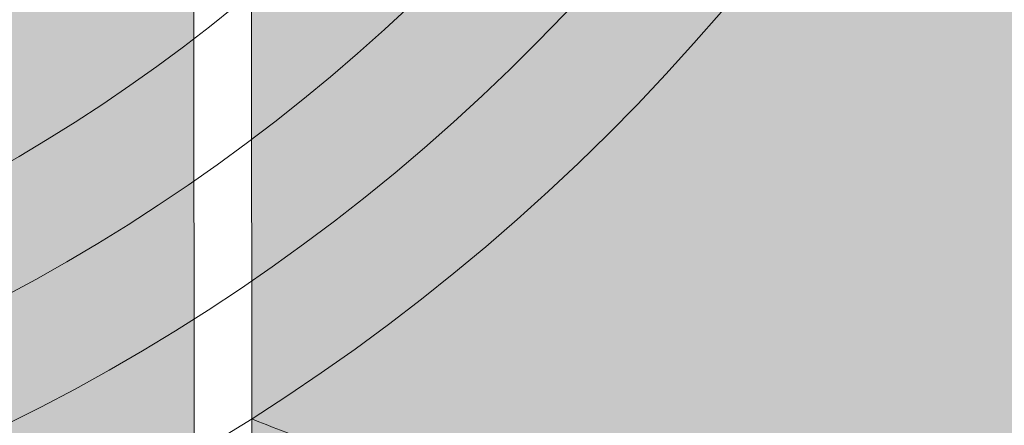
# Model space of a CAD drawing. Units: millimetres. Extents: x 11032 to 26788, y 3406 to 24505.
# Tile 23 of 78: x 18325 to 18753, y 10998 to 11174. Entities that reach past the tile are written whole.
import ezdxf

# ---------------------------------------------------------------- set-up
doc = ezdxf.new("R2010")
doc.units = ezdxf.units.MM
doc.header["$MEASUREMENT"] = 0
for name, color, linetype, lineweight in [('A-ANNO-DIMS', 2, 'Continuous', 18), ('A-ELEV-GUIT', 7, 'Continuous', 18), ('A-ELEV-GUIT-PATT', 7, 'Continuous', 13), ('A-ELEV-INLY', 8, 'Continuous', 13), ('A-ELEV-INLY-PATT', 250, 'Continuous', 13), ('A-ELEV-STRG', 7, 'Continuous', 13)]:
    doc.layers.add(name, color=color, linetype=linetype, lineweight=lineweight)
doc.styles.get("Standard").update_dxf_attribs({"font": 'arial.ttf'})
doc.dimstyles.get("Standard").update_dxf_attribs({"dimtxt": 150, "dimasz": 100, "dimexe": 10, "dimexo": 5, "dimgap": 5, "dimtad": 0, "dimtih": 1, "dimtoh": 1, "dimdec": 0, "dimzin": 0, "dimdsep": 46, "dimtxsty": 'Standard', "dimcen": 0.09, "dimadec": 0, "dimazin": 0, "dimtfac": 1, "dimtdec": 0, "dimtofl": 0, "dimtmove": 0, "dimatfit": 3, "dimfxl": 1, "dimtolj": 1, "dimtzin": 0, "dimarcsym": 0})

# ---------------------------------------------------------------- blocks, each defined once
blk = doc.blocks.new('*D36')
at = {"layer": 'A-ANNO-DIMS', "color": 0, "lineweight": -2, "transparency": 16777216}
for p, q in [((12301.26, 17115.89), (12301.26, 24416.86)), ((25397.4, 4466.4), (25397.4, 24416.86)), ((12401.26, 24406.86), (18569.2, 24406.86)), ((25297.4, 24406.86), (19129.47, 24406.86))]:
    blk.add_line(p, q, dxfattribs=at)
at = {"layer": 'A-ANNO-DIMS', "color": 0, "transparency": 16777216}
for points in [[(12401.26, 24423.52), (12401.26, 24390.19), (12301.26, 24406.86)], [(25297.4, 24423.52), (25297.4, 24390.19), (25397.4, 24406.86)]]:
    blk.add_solid(points, dxfattribs=at)
at = {"layer": 'Defpoints', "color": 0, "transparency": 16777216}
for p in [(25397.4, 24406.86), (12301.26, 17110.89), (25397.4, 4461.4)]:
    blk.add_point(p, dxfattribs=at)
at = {"layer": 'A-ANNO-DIMS', "color": 0, "transparency": 16777216, "insert": (18849.33, 24406.86), "char_height": 150, "attachment_point": 5}
blk.add_mtext('\\A1;13096', dxfattribs=at)
blk = doc.blocks.new('*D50')
at = {"layer": 'A-ANNO-DIMS', "color": 0, "lineweight": -2, "transparency": 16777216}
for p, q in [((19697.4, 16000.71), (19697.4, 3494.9)), ((17953.45, 10206.41), (17953.45, 3494.9)), ((18053.45, 3504.9), (18603.82, 3504.9)), ((19597.4, 3504.9), (19047.04, 3504.9))]:
    blk.add_line(p, q, dxfattribs=at)
at = {"layer": 'A-ANNO-DIMS', "color": 0, "transparency": 16777216}
for points in [[(18053.45, 3521.57), (18053.45, 3488.23), (17953.45, 3504.9)], [(19597.4, 3521.57), (19597.4, 3488.23), (19697.4, 3504.9)]]:
    blk.add_solid(points, dxfattribs=at)
at = {"layer": 'Defpoints', "color": 0, "transparency": 16777216}
for p in [(19697.4, 16005.71), (17953.45, 10211.41), (19697.4, 3504.9)]:
    blk.add_point(p, dxfattribs=at)
at = {"layer": 'A-ANNO-DIMS', "color": 0, "transparency": 16777216, "insert": (18825.43, 3504.9), "char_height": 150, "attachment_point": 5}
blk.add_mtext('\\A1;1744', dxfattribs=at)
blk = doc.blocks.new('*D57')
at = {"layer": 'A-ANNO-DIMS', "color": 0, "lineweight": -2, "transparency": 16777216}
for p, q in [((14994.7, 7266.4), (14994.7, 24416.86)), ((20894.7, 7266.4), (20894.7, 24416.86)), ((15094.7, 24406.86), (17715.98, 24406.86)), ((20794.7, 24406.86), (18173.42, 24406.86))]:
    blk.add_line(p, q, dxfattribs=at)
at = {"layer": 'A-ANNO-DIMS', "color": 0, "transparency": 16777216}
for points in [[(15094.7, 24423.52), (15094.7, 24390.19), (14994.7, 24406.86)], [(20794.7, 24423.52), (20794.7, 24390.19), (20894.7, 24406.86)]]:
    blk.add_solid(points, dxfattribs=at)
at = {"layer": 'Defpoints', "color": 0, "transparency": 16777216}
for p in [(20894.7, 24406.86), (14994.7, 7261.4), (20894.7, 7261.4)]:
    blk.add_point(p, dxfattribs=at)
at = {"layer": 'A-ANNO-DIMS', "color": 0, "transparency": 16777216, "insert": (17944.7, 24406.86), "char_height": 150, "attachment_point": 5}
blk.add_mtext('\\A1;5900', dxfattribs=at)
blk = doc.blocks.new('*D70')
at = {"layer": 'A-ANNO-DIMS', "color": 0, "lineweight": -2, "transparency": 16777216}
for p, q in [((18044.7, 11901.4), (17944.7, 11901.4)), ((17944.7, 11901.4), (17944.7, 10261.4)), ((17944.61, 7261.4), (17944.79, 7261.4)), ((17944.7, 7261.31), (17944.7, 7261.49))]:
    blk.add_line(p, q, dxfattribs=at)
at = {"layer": 'A-ANNO-DIMS', "color": 0, "transparency": 16777216}
blk.add_solid([(17928.04, 10261.4), (17961.37, 10261.4), (17944.7, 10161.4)], dxfattribs=at)
at = {"layer": 'Defpoints', "color": 0, "transparency": 16777216}
for p in [(17944.7, 10161.4), (17944.7, 7261.4)]:
    blk.add_point(p, dxfattribs=at)
at = {"layer": 'A-ANNO-DIMS', "color": 0, "transparency": 16777216, "insert": (18345.2, 11901.4), "char_height": 150, "attachment_point": 5}
blk.add_mtext('\\A1;R2900', dxfattribs=at)
blk = doc.blocks.new('*D78')
at = {"layer": 'A-ANNO-DIMS', "color": 0, "lineweight": -2, "transparency": 16777216}
for p, q in [((19278.06, 11833.8), (19378.06, 11833.8)), ((19378.06, 11833.8), (19386.9, 11238.32)), ((19405.52, 9979.24), (19405.7, 9979.24)), ((19405.61, 9979.15), (19405.61, 9979.33))]:
    blk.add_line(p, q, dxfattribs=at)
at = {"layer": 'A-ANNO-DIMS', "color": 0, "transparency": 16777216}
blk.add_solid([(19403.57, 11238.57), (19370.24, 11238.08), (19388.39, 11138.34)], dxfattribs=at)
at = {"layer": 'Defpoints', "color": 0, "transparency": 16777216}
for p in [(19388.39, 11138.34), (19405.61, 9979.24)]:
    blk.add_point(p, dxfattribs=at)
at = {"layer": 'A-ANNO-DIMS', "color": 0, "transparency": 16777216, "insert": (18728.26, 11833.8), "char_height": 150, "attachment_point": 5}
blk.add_mtext('\\A1;2X R1159.2', dxfattribs=at)
blk = doc.blocks.new('*D79')
at = {"layer": 'A-ANNO-DIMS', "color": 0, "lineweight": -2, "transparency": 16777216}
for p, q in [((19621.6, 11163.41), (19157.07, 10798.82)), ((19721.6, 11163.41), (19621.6, 11163.41)), ((18173, 10026.54), (18173.18, 10026.54)), ((18173.09, 10026.45), (18173.09, 10026.63))]:
    blk.add_line(p, q, dxfattribs=at)
at = {"layer": 'A-ANNO-DIMS', "color": 0, "transparency": 16777216}
blk.add_solid([(19146.78, 10811.93), (19167.36, 10785.71), (19078.4, 10737.08)], dxfattribs=at)
at = {"layer": 'Defpoints', "color": 0, "transparency": 16777216}
for p in [(19078.4, 10737.08), (18173.09, 10026.54)]:
    blk.add_point(p, dxfattribs=at)
at = {"layer": 'A-ANNO-DIMS', "color": 0, "transparency": 16777216, "insert": (20272.31, 11163.41), "char_height": 150, "attachment_point": 5}
blk.add_mtext('\\A1;2X R1150.9', dxfattribs=at)
blk = doc.blocks.new('*D80')
at = {"layer": 'A-ANNO-DIMS', "color": 0, "lineweight": -2, "transparency": 16777216}
for p, q in [((18808.09, 11500), (18908.09, 11500)), ((18908.09, 11500), (19122.53, 11163.36)), ((19623.1, 10377.38), (19623.28, 10377.38)), ((19623.19, 10377.29), (19623.19, 10377.47))]:
    blk.add_line(p, q, dxfattribs=at)
at = {"layer": 'A-ANNO-DIMS', "color": 0, "transparency": 16777216}
blk.add_solid([(19136.58, 11172.31), (19108.47, 11154.4), (19176.25, 11079.02)], dxfattribs=at)
at = {"layer": 'Defpoints', "color": 0, "transparency": 16777216}
for p in [(19176.25, 11079.02), (19623.19, 10377.38)]:
    blk.add_point(p, dxfattribs=at)
at = {"layer": 'A-ANNO-DIMS', "color": 0, "transparency": 16777216, "insert": (18315.64, 11500), "char_height": 150, "attachment_point": 5}
blk.add_mtext('\\A1;2X R831.9', dxfattribs=at)
blk = doc.blocks.new('*D81')
at = {"layer": 'A-ANNO-DIMS', "color": 0, "lineweight": -2, "transparency": 16777216}
for p, q in [((18746.01, 11278.33), (18846.01, 11278.33)), ((18846.01, 11278.33), (19073.46, 10960.86)), ((19607.77, 10214.96), (19607.95, 10214.96)), ((19607.86, 10214.87), (19607.86, 10215.05))]:
    blk.add_line(p, q, dxfattribs=at)
at = {"layer": 'A-ANNO-DIMS', "color": 0, "transparency": 16777216}
blk.add_solid([(19087.01, 10970.56), (19059.91, 10951.15), (19131.7, 10879.56)], dxfattribs=at)
at = {"layer": 'Defpoints', "color": 0, "transparency": 16777216}
for p in [(19131.7, 10879.56), (19607.86, 10214.96)]:
    blk.add_point(p, dxfattribs=at)
at = {"layer": 'A-ANNO-DIMS', "color": 0, "transparency": 16777216, "insert": (18253.76, 11278.33), "char_height": 150, "attachment_point": 5}
blk.add_mtext('\\A1;2X R817.6', dxfattribs=at)
blk = doc.blocks.new('*D83')
at = {"layer": 'A-ANNO-DIMS', "color": 0, "lineweight": -2, "transparency": 16777216}
for p, q in [((19272.33, 11150.07), (19043.23, 10964.72)), ((19372.33, 11150.07), (19272.33, 11150.07)), ((18454.06, 10487.99), (18454.06, 10488.17)), ((18453.97, 10488.08), (18454.15, 10488.08))]:
    blk.add_line(p, q, dxfattribs=at)
at = {"layer": 'A-ANNO-DIMS', "color": 0, "transparency": 16777216}
blk.add_solid([(19032.74, 10977.67), (19053.71, 10951.76), (18965.48, 10901.82)], dxfattribs=at)
at = {"layer": 'Defpoints', "color": 0, "transparency": 16777216}
for p in [(18965.48, 10901.82), (18454.06, 10488.08)]:
    blk.add_point(p, dxfattribs=at)
at = {"layer": 'A-ANNO-DIMS', "color": 0, "transparency": 16777216, "insert": (19864.78, 11150.07), "char_height": 150, "attachment_point": 5}
blk.add_mtext('\\A1;2X R657.8', dxfattribs=at)
blk = doc.blocks.new('*D84')
at = {"layer": 'A-ANNO-DIMS', "color": 0, "lineweight": -2, "transparency": 16777216}
for p, q in [((18888.04, 11434.41), (18988.04, 11434.41)), ((18988.04, 11434.41), (19243.8, 11304.14)), ((19907.6, 10966), (19907.78, 10966)), ((19907.69, 10965.91), (19907.69, 10966.09))]:
    blk.add_line(p, q, dxfattribs=at)
at = {"layer": 'A-ANNO-DIMS', "color": 0, "transparency": 16777216}
blk.add_solid([(19251.37, 11319), (19236.24, 11289.29), (19332.91, 11258.76)], dxfattribs=at)
at = {"layer": 'Defpoints', "color": 0, "transparency": 16777216}
for p in [(19332.91, 11258.76), (19907.69, 10966)]:
    blk.add_point(p, dxfattribs=at)
at = {"layer": 'A-ANNO-DIMS', "color": 0, "transparency": 16777216, "insert": (18482.56, 11434.41), "char_height": 150, "attachment_point": 5}
blk.add_mtext('\\A1;2X R645', dxfattribs=at)
blk = doc.blocks.new('*D85')
at = {"layer": 'A-ANNO-DIMS', "color": 0, "lineweight": -2, "transparency": 16777216}
for p, q in [((19336.15, 10949.98), (19136.5, 10931.99)), ((18538.07, 10878.07), (18538.25, 10878.07)), ((18538.16, 10877.98), (18538.16, 10878.16))]:
    blk.add_line(p, q, dxfattribs=at)
at = {"layer": 'A-ANNO-DIMS', "color": 0, "transparency": 16777216}
blk.add_solid([(19135, 10948.59), (19138, 10915.39), (19036.9, 10923.01)], dxfattribs=at)
at = {"layer": 'Defpoints', "color": 0, "transparency": 16777216}
for p in [(19036.9, 10923.01), (18538.16, 10878.07)]:
    blk.add_point(p, dxfattribs=at)
at = {"layer": 'A-ANNO-DIMS', "color": 0, "transparency": 16777216, "insert": (19828.6, 10949.98), "char_height": 150, "attachment_point": 5}
blk.add_mtext('\\A1;2X R500.8', dxfattribs=at)

msp = doc.modelspace()

# ---------------------------------------------------------------- hatches: boundary and pattern name
at = {"layer": 'A-ELEV-GUIT-PATT'}
h = msp.add_hatch(color=256, dxfattribs=at)
h.paths.add_polyline_path([(18424.39, 12337.941), (18425.299, 11185.614, 0.4683722)])
h.paths.add_polyline_path([(17502.928, 12367.48, 0.4909953), (17469.585, 11181.087)])
h.paths.add_polyline_path([(17654.236, 12452.868, 0.0477145), (17528.428, 12385.27), (17494.045, 11161.894, 0.0503453), (17622.952, 11083.922)])
h.paths.add_polyline_path([(17803.94, 12498.071, 0.0431928), (17679.468, 12462.933), (17647.696, 11072.715, 0.0458241), (17778.106, 11030.137)])
h.paths.add_polyline_path([(17950.249, 12511.239), (17829.354, 12521.528), (17803.014, 11024.905, 0.0436508), (17933.027, 11011.49)])
h.paths.add_polyline_path([(18101.906, 12494.739, 0.0426353), (17975.244, 12510.777), (17958.028, 11011.518, 0.0435176), (18087.619, 11025.142)])
h.paths.add_polyline_path([(18250.372, 12446.284, 0.0436439), (18126.849, 12488.945), (18112.671, 11030.45, 0.0462768), (18244.243, 11073.812)])
h.paths.add_polyline_path([(18399.373, 12357.869, 0.0487365), (18275.32, 12434.595), (18269.295, 11085.277, 0.0513698), (18400.312, 11165.647)])
h = msp.add_hatch(color=256, dxfattribs=at)
h.paths.add_polyline_path([(18424.244, 12523.003), (18424.291, 12463.18, -0.5273141), (18425.397, 11060.376), (18425.445, 11000.552, 0.5515566)])
h.paths.add_polyline_path([(18424.291, 12463.18), (18424.34, 12401.672, -0.4998624), (18425.349, 11121.884), (18425.397, 11060.376, 0.5273141)], flags=17)
h.paths.add_polyline_path([(18424.34, 12401.672), (18424.39, 12337.941, -0.4683722), (18425.299, 11185.614), (18425.349, 11121.884, 0.4998624)], flags=16)
h = msp.add_hatch(color=256, dxfattribs=at)
h.paths.add_polyline_path([(18400.408, 11043.88, -0.0436878), (18268.805, 10975.614), (18268.564, 10921.688, 0.0407453), (18400.454, 10985.325)])
h.paths.add_polyline_path([(18243.761, 10965.745, -0.0404734), (18111.675, 10927.96), (18111.179, 10876.93, 0.038119), (18243.523, 10912.454)])
h.paths.add_polyline_path([(18086.629, 10923.332, -0.0383771), (17956.879, 10911.486), (17956.305, 10861.474, 0.0362436), (18086.136, 10872.581)])
h.paths.add_polyline_path([(17931.879, 10911.496, -0.0386479), (17801.231, 10923.595), (17800.341, 10873.053, 0.0365688), (17931.305, 10861.499)])
h.paths.add_polyline_path([(17776.312, 10928.246, -0.0401698), (17645.255, 10965.893), (17644.048, 10913.103, 0.037865), (17775.419, 10877.463)])
h.paths.add_polyline_path([(17490.698, 11042.804), (17489.08, 10985.25, 0.0402314), (17619.258, 10922.301), (17620.478, 10975.665, -0.0430555)])
h.paths.add_polyline_path([(17492.349, 11101.569), (17490.698, 11042.804, 0.0430555), (17620.478, 10975.665), (17621.708, 11029.502, -0.0463742)])
h.paths.add_polyline_path([(17622.952, 11083.922, -0.0503453), (17494.045, 11161.894), (17492.349, 11101.569, 0.0463742), (17621.708, 11029.502)])
h.paths.add_polyline_path([(17647.696, 11072.715), (17646.47, 11019.067, 0.0427975), (17777.208, 10979.13), (17778.106, 11030.137, -0.0458241)])
h.paths.add_polyline_path([(17777.208, 10979.13, -0.0427975), (17646.47, 11019.067), (17645.255, 10965.893, 0.0401698), (17776.312, 10928.246)])
h.paths.add_polyline_path([(17932.453, 10961.493, -0.0409906), (17802.122, 10974.208), (17801.231, 10923.595, 0.0386479), (17931.879, 10911.496)])
h.paths.add_polyline_path([(17933.027, 11011.49, -0.0436508), (17803.014, 11024.905), (17802.122, 10974.208, 0.0409906), (17932.453, 10961.493)])
h.paths.add_polyline_path([(18087.619, 11025.142, -0.0435176), (17958.028, 11011.518), (17957.453, 10961.501, 0.040783), (18087.124, 10974.178)])
h.paths.add_polyline_path([(18087.124, 10974.178, -0.040783), (17957.453, 10961.501), (17956.879, 10911.486, 0.0383771), (18086.629, 10923.332)])
h.paths.add_polyline_path([(18243.761, 10965.745), (18244.001, 11019.495, -0.0431653), (18112.172, 10979.124), (18111.675, 10927.96, 0.0404734)])
h.paths.add_polyline_path([(18244.243, 11073.812, -0.0462768), (18112.671, 11030.45), (18112.172, 10979.124, 0.0431653), (18244.001, 11019.495)])
h.paths.add_polyline_path([(18400.361, 11103.846), (18400.312, 11165.647, -0.0513698), (18269.295, 11085.277), (18269.048, 11030.099, 0.0471686)])
h.paths.add_polyline_path([(18400.361, 11103.846, -0.0471686), (18269.048, 11030.099), (18268.805, 10975.614, 0.0436878), (18400.408, 11043.88)])
at = {"layer": 'A-ELEV-INLY-PATT'}
h = msp.add_hatch(color=256, dxfattribs=at)
h.set_gradient(color2=(38, 38, 39), name='HEMISPHERICAL')
edge = h.paths.add_edge_path()
edge.add_spline(control_points=[(18425.445, 11000.552), (18458.708, 10987.38), (18550.3, 10951.111), (18655.663, 10967.984), (18775.66, 10985.753), (18767.173, 11045.69), (18820.435, 11029.121), (18856.601, 11081.429), (18910.606, 10999.748), (18944.51, 11067.805), (18993.671, 11025.073), (19010.479, 11088.113), (19112.886, 11074.83), (18997.512, 11168.165), (19020.085, 11271.149), (19186.417, 11251.458), (19043.711, 11367.761), (19195.966, 11319.856), (19164.81, 11418.359), (19240.548, 11369.352), (19291.772, 11465.595), (19340.205, 11366.103), (19400.937, 11422.431), (19448.16, 11354.501), (19470.028, 11298.294), (19504.824, 11295.807)], knot_values=[0, 0, 0, 0, 104.1926844, 286.8965309, 358.0276019, 380.9077181, 428.8178922, 462.9108054, 536.6618053, 575.7062143, 616.0072998, 661.1892288, 710.1041052, 826.2545772, 880.3446099, 992.4558514, 1059.8900815, 1142.5885686, 1188.5458396, 1228.1561193, 1314.4611862, 1376.292047, 1433.035567, 1479.0146796, 1584.2445291, 1584.2445291, 1584.2445291, 1584.2445291], degree=3, periodic=0)
edge.add_spline(control_points=[(19504.824, 11295.807), (19505.924, 11314.349), (19506.623, 11332.908), (19508.291, 11422.259), (19504.403, 11492.427), (19485.077, 11629.54), (19469.639, 11696.485), (19436.971, 11793.081), (19424.498, 11824.643), (19403.303, 11870.856), (19395.824, 11886.073), (19380.021, 11916.101), (19371.692, 11930.911), (19325.511, 12008.031), (19280.532, 12066.689), (19204.455, 12147.807), (19177.661, 12173.701), (19101.242, 12241.001), (19049.213, 12279.949), (18967.517, 12332.138), (18939.676, 12348.496), (18883.071, 12379.019), (18854.309, 12393.182), (18810.69, 12412.702), (18796.068, 12418.926), (18764.062, 12431.927), (18746.648, 12438.606), (18662.541, 12469.232), (18594.628, 12489.063), (18492.28, 12515.967), (18458.285, 12524.419), (18424.236, 12532.741)], knot_values=[45.1275191, 45.1275191, 45.1275191, 45.1275191, 98.76835, 98.76835, 303.9642424, 303.9642424, 509.1601349, 509.1601349, 611.7580811, 611.7580811, 663.0570542, 663.0570542, 714.3560273, 714.3560273, 934.0138233, 934.0138233, 1043.8427213, 1043.8427213, 1233.750961, 1233.750961, 1328.7050808, 1328.7050808, 1423.6592007, 1423.6592007, 1471.1362606, 1471.1362606, 1527.0566313, 1527.0566313, 1739.8301307, 1739.8301307, 1844.9911016, 1844.9911016, 1844.9911016, 1844.9911016], degree=3, periodic=0)
edge.add_line((18424.236, 12532.741), (18424.244, 12523.003))
edge.add_arc((17944.704, 11761.399), 900, -57.713267, 57.803626, ccw=False)
h = msp.add_hatch(color=256, dxfattribs=at)
edge = h.paths.add_edge_path()
edge.add_line((18641.912, 10936.669), (18683.084, 10885.205))
edge.add_line((18683.084, 10885.205), (18707.528, 10942.241))
edge.add_line((18707.528, 10942.241), (18707.585, 10942.062))
edge.add_line((18707.585, 10942.062), (18728.977, 10934.931))
edge.add_line((18728.977, 10934.931), (18746.506, 10952.29))
edge.add_line((18746.506, 10952.29), (18731.852, 10933.973))
edge.add_line((18731.852, 10933.973), (18772.392, 10896.329))
edge.add_line((18772.392, 10896.329), (18806.063, 10924.18))
edge.add_line((18806.063, 10924.18), (18807.011, 10949.111))
edge.add_line((18807.011, 10949.111), (18828.079, 10974.85))
edge.add_line((18828.079, 10974.85), (18819.406, 10935.218))
edge.add_line((18819.406, 10935.218), (18806.063, 10924.18))
edge.add_line((18806.063, 10924.18), (18804.745, 10889.526))
edge.add_line((18804.745, 10889.526), (18898.625, 10928.045))
edge.add_line((18898.625, 10928.045), (18869.346, 10974.891))
edge.add_line((18869.346, 10974.891), (18881.224, 11043.454))
edge.add_spline(control_points=[(18881.224, 11043.454), (18869.883, 11051.959), (18847.69, 11068.541), (18820.435, 11029.121), (18767.173, 11045.69), (18775.66, 10985.753), (18655.663, 10967.984), (18550.3, 10951.111), (18458.708, 10987.38), (18425.445, 11000.552)], knot_values=[0, 0, 0, 0, 35.3761266, 69.4690398, 117.3792138, 140.25933, 211.3904011, 394.0942475, 498.2869319, 498.2869319, 498.2869319, 498.2869319], degree=3, periodic=0)
edge.add_line((18425.445, 11000.552), (18425.52, 10905.025))
edge.add_line((18425.52, 10905.025), (18430.245, 10896.05))
edge.add_line((18430.245, 10896.05), (18435.033, 10901.9))
edge.add_line((18435.033, 10901.9), (18426.36, 10862.267))
edge.add_line((18426.36, 10862.267), (18425.554, 10861.6))
edge.add_line((18425.554, 10861.6), (18425.592, 10814.001))
edge.add_spline(control_points=[(18425.592, 10814.001), (18433.789, 10803.871), (18442.268, 10794.033), (18451.048, 10784.539)], knot_values=[3268.8603349, 3268.8603349, 3268.8603349, 3268.8603349, 3307.7959894, 3307.7959894, 3307.7959894, 3307.7959894], degree=3, periodic=0)
edge.add_line((18451.048, 10784.539), (18509.494, 10848.83))
edge.add_line((18509.494, 10848.83), (18582.646, 10885.406))
edge.add_line((18582.646, 10885.406), (18583.089, 10886.145))
edge.add_line((18583.089, 10886.145), (18587.289, 10850.746))
edge.add_line((18587.289, 10850.746), (18609.162, 10818.698))
edge.add_line((18609.162, 10818.698), (18619.222, 10824.446))
edge.add_line((18619.222, 10824.446), (18621.931, 10828.059))
edge.add_line((18621.931, 10828.059), (18609.651, 10885.365))
edge.add_line((18609.651, 10885.365), (18631.427, 10872.922))
edge.add_line((18631.427, 10872.922), (18641.912, 10936.669))
edge = h.paths.add_edge_path()
edge.add_spline(control_points=[(18521.786, 10715.217), (18494.865, 10734.264), (18470.266, 10756.433), (18447.672, 10780.825)], knot_values=[3169.2083247, 3169.2083247, 3169.2083247, 3169.2083247, 3268.4288812, 3268.4288812, 3268.4288812, 3268.4288812], degree=3, periodic=0)
edge.add_line((18447.672, 10780.825), (18509.494, 10848.83))
edge.add_line((18509.494, 10848.83), (18553.129, 10870.647))
edge.add_line((18553.129, 10870.647), (18595.722, 10811.017))
edge.add_line((18595.722, 10811.017), (18533.878, 10775.678))
edge.add_line((18533.878, 10775.678), (18521.786, 10715.217))
h.paths.add_polyline_path([(18605.498, 10816.604), (18533.878, 10775.678), (18531.124, 10761.907), (18641.898, 10699.586), (18643.606, 10726.91), (18634.217, 10770.728)])
edge = h.paths.add_edge_path()
edge.add_line((18785.911, 10769.68), (18741.142, 10702.526))
edge.add_line((18741.142, 10702.526), (18708.511, 10675.334))
edge.add_line((18708.511, 10675.334), (18722.102, 10641.355))
edge.add_spline(control_points=[(18722.102, 10641.355), (18731.823, 10639.718), (18741.633, 10638.316), (18776.029, 10634.243), (18801.002, 10632.764), (18826.213, 10632.653)], knot_values=[2859.5985359, 2859.5985359, 2859.5985359, 2859.5985359, 2887.7863004, 2887.7863004, 2957.6673477, 2957.6673477, 2957.6673477, 2957.6673477], degree=3, periodic=0)
edge.add_line((18826.213, 10632.653), (18785.911, 10769.68))
h.paths.add_polyline_path([(18731.852, 10933.973), (18728.977, 10934.931), (18717.029, 10923.099), (18711.602, 10884.111), (18717.158, 10823.933), (18748.841, 10805.828), (18750.362, 10810.578), (18809.167, 10862.181)], flags=17)
h.paths.add_polyline_path([(18718.941, 10804.621), (18683.084, 10820.92), (18683.084, 10787.669), (18707.124, 10679.488), (18725.547, 10733.082)])
h.paths.add_polyline_path([(18683.084, 10820.92), (18647.71, 10836.999), (18643.606, 10800.062), (18672.952, 10719.36), (18706.848, 10678.685), (18707.124, 10679.488), (18683.084, 10787.669)])
edge = h.paths.add_edge_path()
edge.add_arc((19371.815, 10038.476), 831.89, 122.374168, 124.844789)
edge.add_line((18896.51, 10721.211), (18891.739, 10678.265))
edge.add_line((18891.739, 10678.265), (18894.756, 10635.646))
edge.add_spline(control_points=[(18894.756, 10635.646), (18903.281, 10636.419), (18911.81, 10637.341), (18928.187, 10639.393), (18936.036, 10640.501), (18943.874, 10641.731)], knot_values=[2751.6881001, 2751.6881001, 2751.6881001, 2751.6881001, 2775.0905103, 2775.0905103, 2796.6501133, 2796.6501133, 2796.6501133, 2796.6501133], degree=3, periodic=0)
edge.add_line((18943.874, 10641.731), (18941.931, 10680.282))
edge.add_line((18941.931, 10680.282), (18939.116, 10690.133))
edge.add_line((18939.116, 10690.133), (18926.383, 10741.065))
h.paths.add_polyline_path([(18809.167, 10862.181), (18750.362, 10810.578), (18748.841, 10805.828), (18780.62, 10787.669), (18798.474, 10726.964), (18899.548, 10748.547), (18902.54, 10775.477)])
h.paths.add_polyline_path([(19113.073, 10865.816), (19104.648, 10957.062), (19105.426, 10962.649, 0.0520192), (19048.031, 10841.722), (19056.443, 10818.589, -0.0225594)])
edge = h.paths.add_edge_path()
edge.add_spline(control_points=[(19487.22, 11152.261), (19488.987, 11161.344), (19490.621, 11170.471), (19492.803, 11183.73), (19493.451, 11187.834), (19494.075, 11191.944)], knot_values=[1945.7202792, 1945.7202792, 1945.7202792, 1945.7202792, 1972.729714, 1972.729714, 1984.803134, 1984.803134, 1984.803134, 1984.803134], degree=3, periodic=0)
edge.add_spline(control_points=[(19494.075, 11191.944), (19496.769, 11209.693), (19499, 11227.566), (19500.813, 11245.508)], knot_values=[1893.583377, 1893.583377, 1893.583377, 1893.583377, 1945.7202792, 1945.7202792, 1945.7202792, 1945.7202792], degree=3, periodic=0)
edge.add_line((19500.813, 11245.508), (19455.113, 11264.581))
edge.add_arc((19859.228, 10553.861), 817.577, 119.622547, 134.325807)
edge.add_arc((19623.186, 10377.382), 831.89, 113.764176, 113.962715)
edge.add_arc((18705.433, 10826.987), 657.823, 27.671781, 28.173232, ccw=False)
edge.add_arc((19405.609, 9979.237), 1159.227, 86.129259, 95.822157, ccw=False)
edge.add_spline(control_points=[(19483.864, 11135.82), (19485.032, 11141.283), (19486.15, 11146.764), (19487.22, 11152.261)], knot_values=[1984.803134, 1984.803134, 1984.803134, 1984.803134, 2001.1514712, 2001.1514712, 2001.1514712, 2001.1514712], degree=3, periodic=0)

# ---------------------------------------------------------------- linework, layer by layer
at = {"layer": 'A-ELEV-GUIT'}
for radius, start, end in [(900, 118.96712, 57.803626), (850, 121.044036, 55.651805), (800, 123.369805, 53.162671), (750, 126.088521, 50.239355)]:
    msp.add_arc((17944.704, 11761.399), radius, start, end, dxfattribs=at)
at = {"layer": 'A-ELEV-INLY'}
for points, knots in [([(18424.232, 12537.889), (18562.977, 12503.994), (18939.42, 12405.671), (19429.901, 11996.89), (19551.657, 11366.066), (19406.266, 10676.866), (18611.174, 10531.068), (18382.465, 10854.626), (18332.323, 10949.148)], [43.9017403, 43.9017403, 43.9017403, 43.9017403, 472.2498304, 1211.2844307, 1793.6258437, 2340.5272824, 3154.1000811, 3469.5948326, 3469.5948326, 3469.5948326, 3469.5948326]), ([(18423.046, 12533.032), (18457.492, 12524.616), (18491.885, 12516.07), (18594.628, 12489.063), (18662.541, 12469.232), (18746.648, 12438.606), (18764.062, 12431.927), (18796.068, 12418.926), (18810.69, 12412.702), (18854.309, 12393.182), (18883.071, 12379.019), (18939.676, 12348.496), (18967.517, 12332.138), (19049.213, 12279.949), (19101.242, 12241.001), (19177.661, 12173.701), (19204.455, 12147.807), (19280.532, 12066.689), (19325.511, 12008.031), (19371.692, 11930.911), (19380.021, 11916.101), (19395.824, 11886.073), (19403.303, 11870.856), (19424.498, 11824.643), (19436.971, 11793.081), (19469.639, 11696.485), (19485.077, 11629.54), (19504.403, 11492.427), (19508.291, 11422.259), (19505.897, 11293.968), (19501.419, 11236.104), (19482.838, 11123.165), (19468.734, 11068.091), (19432.486, 10975.468), (19412.727, 10936.698), (19380.78, 10889.312), (19372.633, 10878.181), (19356.856, 10858.373), (19349.373, 10849.6), (19334.153, 10832.974), (19326.448, 10825.097), (19310.441, 10809.758), (19302.142, 10802.295), (19276.431, 10780.55), (19258.2, 10766.907), (19193.085, 10723.572), (19141.86, 10698.191), (19033.937, 10659.174), (18977.24, 10645.539), (18863.428, 10631.28), (18806.315, 10630.657), (18706.774, 10642.444), (18663.576, 10652.483), (18610.301, 10672.44), (18597.617, 10677.83), (18575.274, 10688.559), (18565.496, 10693.716), (18548.658, 10703.464), (18541.496, 10707.907), (18527.484, 10717.221), (18520.632, 10722.092), (18500.516, 10737.302), (18487.695, 10748.238), (18442.023, 10791.459), (18412.68, 10828.089), (18368.505, 10894.404), (18351.99, 10922.743), (18336.74, 10951.492)], [43.9017403, 43.9017403, 43.9017403, 43.9017403, 150.28849, 150.28849, 363.0619895, 363.0619895, 418.9823602, 418.9823602, 466.4594201, 466.4594201, 561.4135399, 561.4135399, 656.3676597, 656.3676597, 846.2758994, 846.2758994, 956.1047974, 956.1047974, 1175.7625934, 1175.7625934, 1227.0615665, 1227.0615665, 1278.3605397, 1278.3605397, 1380.9584859, 1380.9584859, 1586.1543783, 1586.1543783, 1791.3502707, 1791.3502707, 1957.7936992, 1957.7936992, 2124.2371277, 2124.2371277, 2254.8585156, 2254.8585156, 2296.2963307, 2296.2963307, 2330.692619, 2330.692619, 2363.21545, 2363.21545, 2395.7382809, 2395.7382809, 2460.7839427, 2460.7839427, 2617.0158229, 2617.0158229, 2773.247703, 2773.247703, 2929.4795832, 2929.4795832, 3057.0589812, 3057.0589812, 3098.1793964, 3098.1793964, 3131.5312179, 3131.5312179, 3157.1289484, 3157.1289484, 3182.7266789, 3182.7266789, 3233.9221399, 3233.9221399, 3373.2453482, 3373.2453482, 3469.5948326, 3469.5948326, 3469.5948326, 3469.5948326]), ([(18425.445, 11000.552), (18458.708, 10987.38), (18550.3, 10951.111), (18655.663, 10967.984), (18775.66, 10985.753), (18767.173, 11045.69), (18820.435, 11029.121), (18856.601, 11081.429), (18910.606, 10999.748), (18944.51, 11067.805), (18993.671, 11025.073), (19010.479, 11088.113), (19112.886, 11074.83), (18997.512, 11168.165), (19020.085, 11271.149), (19186.417, 11251.458), (19043.711, 11367.761), (19195.966, 11319.856), (19164.81, 11418.359), (19240.548, 11369.352), (19291.772, 11465.595), (19340.205, 11366.103), (19400.937, 11422.431), (19448.16, 11354.501), (19470.283, 11297.639), (19505.995, 11295.734), (19506.584, 11295.703)], [0, 0, 0, 0, 104.1926844, 286.8965309, 358.0276019, 380.9077181, 428.8178922, 462.9108054, 536.6618053, 575.7062143, 616.0072998, 661.1892288, 710.1041052, 826.2545772, 880.3446099, 992.4558514, 1059.8900815, 1142.5885686, 1188.5458396, 1228.1561193, 1314.4611862, 1376.292047, 1433.035567, 1479.0146796, 1584.2445291, 1586.0071764, 1586.0071764, 1586.0071764, 1586.0071764])]:
    msp.add_open_spline(points, degree=3, knots=knots, dxfattribs=at)
at = {"layer": 'A-ELEV-STRG'}
for p, q in [((18400.876, 10451.016), (18391.999, 21713.011)), ((18425.878, 10451.016), (18416.998, 21712.995))]:
    msp.add_line(p, q, dxfattribs=at)

# ---------------------------------------------------------------- dimensions: what is measured, and where the dimension line sits
at = {"layer": 'A-ANNO-DIMS'}
for base, p1, p2, picture, middle in [((25397.404, 24406.858), (12301.265, 17110.885), (25397.404, 4461.399), '*D36', (18849.334, 24406.858)), ((20894.704, 24406.858), (14994.704, 7261.399), (20894.704, 7261.399), '*D57', (17944.704, 24406.858)), ((19697.404, 3504.899), (17953.455, 10211.41), (19697.404, 16005.71), '*D50', (18825.429, 3504.899))]:
    dim = msp.add_linear_dim(base=base, p1=p1, p2=p2, dimstyle='Standard', override={"dimdec": 0, "dimlfac": 1, "dimrnd": 0, "dimzin": 0, "dimdsep": 46, "dimlunit": 2}, dxfattribs=at)
    dim.commit()
    dim.dimension.update_dxf_attribs({"geometry": picture, "text_midpoint": middle})
for center, mpoint, override, picture, middle in [((19405.609, 9979.237), (19388.388, 11138.336), {"dimdec": 1, "dimlfac": 1, "dimrnd": 0, "dimzin": 0, "dimdsep": 46, "dimlunit": 2}, '*D78', (18728.256, 11833.796)), ((19623.186, 10377.382), (19176.251, 11079.016), {"dimdec": 1, "dimlfac": 1, "dimrnd": 0, "dimzin": 0, "dimdsep": 46, "dimlunit": 2}, '*D80', (18315.641, 11499.997)), ((19907.691, 10966.001), (19332.909, 11258.758), {"dimdec": 0, "dimlfac": 1, "dimrnd": 0, "dimzin": 0, "dimdsep": 46, "dimlunit": 2}, '*D84', (18482.562, 11434.412)), ((19607.858, 10214.955), (19131.7, 10879.565), {"dimdec": 1, "dimlfac": 1, "dimrnd": 0, "dimzin": 0, "dimdsep": 46, "dimlunit": 2}, '*D81', (18253.761, 11278.331)), ((18173.088, 10026.538), (19078.405, 10737.081), {"dimdec": 1, "dimlfac": 1, "dimrnd": 0, "dimzin": 0, "dimdsep": 46, "dimlunit": 2}, '*D79', (20272.315, 11163.407)), ((18454.063, 10488.082), (18965.483, 10901.822), {"dimdec": 1, "dimlfac": 1, "dimrnd": 0, "dimzin": 0, "dimdsep": 46, "dimlunit": 2}, '*D83', (19864.784, 11150.066)), ((18538.162, 10878.073), (19036.903, 10923.013), {"dimdec": 1, "dimlfac": 1, "dimrnd": 0, "dimzin": 0, "dimdsep": 46, "dimlunit": 2}, '*D85', (19336.147, 10949.977))]:
    dim = msp.add_radius_dim(center=center, mpoint=mpoint, text='2X <>', dimstyle='Standard', override=override, dxfattribs=at)
    dim.commit()
    dim.dimension.update_dxf_attribs({"geometry": picture, "text_midpoint": middle, "dimtype": 164})
dim = msp.add_radius_dim(center=(17944.704, 7261.399), mpoint=(17944.704, 10161.399), dimstyle='Standard', override={"dimdec": 0, "dimlfac": 1, "dimrnd": 0, "dimzin": 0, "dimdsep": 46, "dimlunit": 2}, dxfattribs=at)
dim.commit()
dim.dimension.update_dxf_attribs({"geometry": '*D70', "text_midpoint": (18345.202, 11901.399), "dimtype": 164})

doc.saveas('drawing.dxf')
